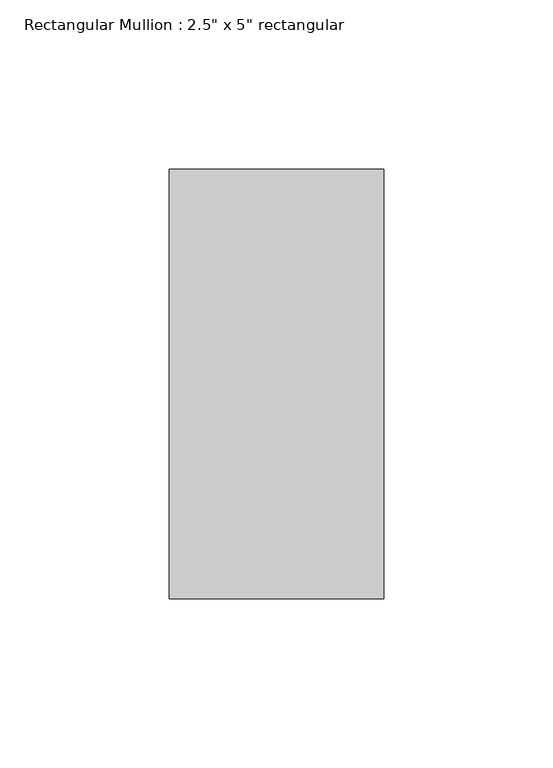
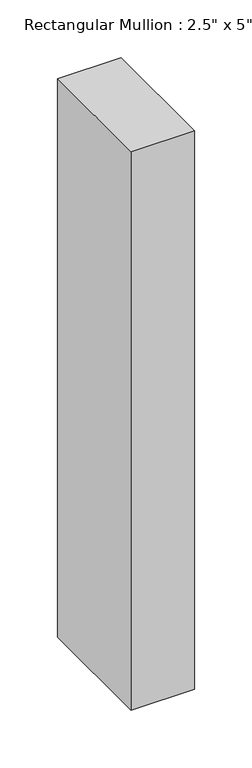
"""IFC4 building model written with IfcOpenShell, lengths in millimetres: member geometry."""

from ifc_helpers import new_model, si_unit, frame, origin, place, context, project, spatial, polyline, outline, extrude, source, transform, mapped, element, save


def member_e5d39754(model_context):
    return source(origin(), model_context, "Body", "SweptSolid", [
        extrude(outline(polyline([(0.0, 63.5), (0.0, -63.5), (-63.5, -63.5), (-63.5, 63.5), (0.0, 63.5)])), frame((0.0, 0.0, -590.55), z_axis=(0.0, 0.0, 1.0), x_axis=(1.0, 0.0, 0.0)), (0.0, 0.0, 1.0), 590.55),
    ])


if __name__ == "__main__":
    model = new_model("IFC4")
    model_context = context("Model", 3, world=origin())
    ifc_project = project(units=[si_unit("LENGTHUNIT", "METRE", prefix="MILLI")], contexts=[model_context])
    site = spatial("IfcSite", under=ifc_project)
    building = spatial("IfcBuilding", under=site)
    placement = place(None, origin())
    member_shape = member_e5d39754(model_context)
    element("IfcMember", 1, ObjectType="Rectangular Mullion : 2.5\" x 5\" rectangular", at=placement, inside=building, context=model_context, shape_type="MappedRepresentation", body=[
        mapped(member_shape, transform((0.0, 0.0, 0.0), x_axis=(1.0, 0.0, 0.0), y_axis=(0.0, 1.0, 0.0), z_axis=(0.0, 0.0, 1.0))),
    ])
    save(model, "model.ifc")

# Revit data of these elements
# Type "Rectangular Mullion : 2.5\" x 5\" rectangular"
#   built-in parameter 1007304 = 0.416667 (stored number, unit not read)
#   built-in parameter 1007301 = 0.104167 (stored number, unit not read)
#   built-in parameter 1007300 = 0.104167 (stored number, unit not read)
# Element 1 (IfcMember, "Rectangular Mullion : 2.5\" x 5\" rectangular")
#   Materials on its faces: "door black"
# Materials
#   "door black": class "Generic", colour RGB 120 120 120, transparency 0, Cost = 0
